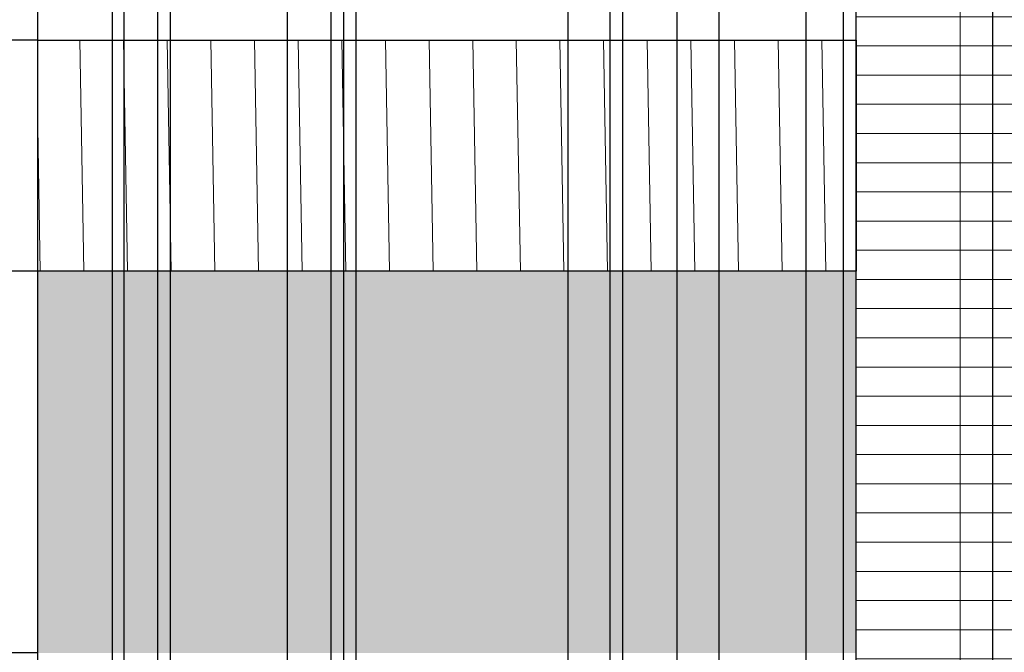
# Model space of a CAD drawing. Units: inches. Extents: x 241 to 943, y 109 to 1396.
# Tile 24 of 34: x 374 to 532, y 1178 to 1279. Entities that reach past the tile are written whole.
import ezdxf

# ---------------------------------------------------------------- set-up
doc = ezdxf.new("R2010")
doc.units = ezdxf.units.IN
doc.header["$MEASUREMENT"] = 0
for name, color, linetype, lineweight in [('A-ANNO-DIMS', 2, 'Continuous', 18), ('A-ELEV', 7, 'Continuous', 25), ('A-ELEV-SHAD', 9, 'Continuous', 13), ('A-WALL-PATT', 8, 'Continuous', 13)]:
    doc.layers.add(name, color=color, linetype=linetype, lineweight=lineweight)
doc.styles.get("Standard").update_dxf_attribs({"font": 'arial.ttf'})
doc.dimstyles.get("Standard").update_dxf_attribs({"dimtxt": 1.4375, "dimasz": 0.18, "dimexe": 0.18, "dimexo": 0.0625, "dimgap": 0.09, "dimtad": 0, "dimtih": 1, "dimtoh": 1, "dimdec": 4, "dimzin": 0, "dimdsep": 46, "dimlunit": 4, "dimtxsty": 'Standard', "dimcen": 0.09, "dimadec": 0, "dimazin": 0, "dimtfac": 1, "dimtdec": 4, "dimtofl": 0, "dimtmove": 0, "dimatfit": 3, "dimfxl": 1, "dimtolj": 1, "dimtzin": 0, "dimarcsym": 0})

# ---------------------------------------------------------------- blocks, each defined once
blk = doc.blocks.new('*D5')
at = {"layer": 'A-ANNO-DIMS', "color": 0, "lineweight": -2, "transparency": 16777216}
for p, q in [((303.24, 177.8), (303.24, 1395.05)), ((303.42, 1394.87), (338.18, 1394.87)), ((376.86, 1394.87), (342.09, 1394.87)), ((377.04, 177.76), (377.04, 1395.05))]:
    blk.add_line(p, q, dxfattribs=at)
at = {"layer": 'A-ANNO-DIMS', "color": 0, "transparency": 16777216}
for points in [[(303.42, 1394.9), (303.42, 1394.84), (303.24, 1394.87)], [(376.86, 1394.9), (376.86, 1394.84), (377.04, 1394.87)]]:
    blk.add_solid(points, dxfattribs=at)
at = {"layer": 'Defpoints', "color": 0, "transparency": 16777216}
for p in [(377.04, 1394.87), (303.24, 177.74), (377.04, 177.7)]:
    blk.add_point(p, dxfattribs=at)
at = {"layer": 'A-ANNO-DIMS', "color": 0, "transparency": 16777216, "insert": (340.14, 1394.87), "char_height": 1.438, "attachment_point": 5}
blk.add_mtext('\\A1;73.8', dxfattribs=at)
blk = doc.blocks.new('*D7')
at = {"layer": 'A-ANNO-DIMS', "color": 0, "lineweight": -2, "transparency": 16777216}
for p, q in [((508.24, 1336.12), (244.31, 1336.12)), ((244.49, 1335.94), (244.49, 753.25)), ((244.49, 168.92), (244.49, 751.6)), ((303.17, 168.74), (244.31, 168.74))]:
    blk.add_line(p, q, dxfattribs=at)
at = {"layer": 'A-ANNO-DIMS', "color": 0, "transparency": 16777216}
for points in [[(244.46, 1335.94), (244.52, 1335.94), (244.49, 1336.12)], [(244.46, 168.92), (244.52, 168.92), (244.49, 168.74)]]:
    blk.add_solid(points, dxfattribs=at)
at = {"layer": 'Defpoints', "color": 0, "transparency": 16777216}
for p in [(244.49, 1336.12), (508.31, 1336.12), (303.24, 168.74)]:
    blk.add_point(p, dxfattribs=at)
at = {"layer": 'A-ANNO-DIMS', "color": 0, "transparency": 16777216, "insert": (244.49, 752.43), "char_height": 1.438, "attachment_point": 5}
blk.add_mtext('\\A1;1167.4', dxfattribs=at)
blk = doc.blocks.new('*D8')
at = {"layer": 'A-ANNO-DIMS', "color": 0, "lineweight": -2, "transparency": 16777216}
for p, q in [((377.04, 396.94), (377.04, 1395.05)), ((377.22, 1394.87), (380.96, 1394.87)), ((390.71, 1394.87), (386.97, 1394.87)), ((390.89, 384.24), (390.89, 1395.05))]:
    blk.add_line(p, q, dxfattribs=at)
at = {"layer": 'A-ANNO-DIMS', "color": 0, "transparency": 16777216}
for points in [[(377.22, 1394.9), (377.22, 1394.84), (377.04, 1394.87)], [(390.71, 1394.9), (390.71, 1394.84), (390.89, 1394.87)]]:
    blk.add_solid(points, dxfattribs=at)
at = {"layer": 'Defpoints', "color": 0, "transparency": 16777216}
for p in [(390.89, 1394.87), (377.04, 396.88), (390.89, 384.18)]:
    blk.add_point(p, dxfattribs=at)
at = {"layer": 'A-ANNO-DIMS', "color": 0, "transparency": 16777216, "insert": (383.97, 1394.87), "char_height": 1.438, "attachment_point": 5}
blk.add_mtext('\\A1;13.856', dxfattribs=at)
blk = doc.blocks.new('*D9')
at = {"layer": 'A-ANNO-DIMS', "color": 0, "lineweight": -2, "transparency": 16777216}
for p, q in [((390.89, 384.24), (390.89, 1395.05)), ((391.07, 1394.87), (424.13, 1394.87)), ((461.93, 1394.87), (428.87, 1394.87)), ((462.11, 384.24), (462.11, 1395.05))]:
    blk.add_line(p, q, dxfattribs=at)
at = {"layer": 'A-ANNO-DIMS', "color": 0, "transparency": 16777216}
for points in [[(391.07, 1394.9), (391.07, 1394.84), (390.89, 1394.87)], [(461.93, 1394.9), (461.93, 1394.84), (462.11, 1394.87)]]:
    blk.add_solid(points, dxfattribs=at)
at = {"layer": 'Defpoints', "color": 0, "transparency": 16777216}
for p in [(462.11, 1394.87), (390.89, 384.18), (462.11, 384.18)]:
    blk.add_point(p, dxfattribs=at)
at = {"layer": 'A-ANNO-DIMS', "color": 0, "transparency": 16777216, "insert": (426.5, 1394.87), "char_height": 1.438, "attachment_point": 5}
blk.add_mtext('\\A1;71.21', dxfattribs=at)
blk = doc.blocks.new('*D10')
at = {"layer": 'A-ANNO-DIMS', "color": 0, "lineweight": -2, "transparency": 16777216}
for p, q in [((462.11, 384.24), (462.11, 1395.05)), ((462.29, 1394.87), (468.4, 1394.87)), ((479.42, 1394.87), (473.3, 1394.87)), ((479.6, 384.24), (479.6, 1395.05))]:
    blk.add_line(p, q, dxfattribs=at)
at = {"layer": 'A-ANNO-DIMS', "color": 0, "transparency": 16777216}
for points in [[(462.29, 1394.9), (462.29, 1394.84), (462.11, 1394.87)], [(479.42, 1394.9), (479.42, 1394.84), (479.6, 1394.87)]]:
    blk.add_solid(points, dxfattribs=at)
at = {"layer": 'Defpoints', "color": 0, "transparency": 16777216}
for p in [(479.6, 1394.87), (462.11, 384.18), (479.6, 384.18)]:
    blk.add_point(p, dxfattribs=at)
at = {"layer": 'A-ANNO-DIMS', "color": 0, "transparency": 16777216, "insert": (470.85, 1394.87), "char_height": 1.438, "attachment_point": 5}
blk.add_mtext('\\A1;17.49', dxfattribs=at)
blk = doc.blocks.new('*D11')
at = {"layer": 'A-ANNO-DIMS', "color": 0, "lineweight": -2, "transparency": 16777216}
for p, q in [((500.33, 384.24), (500.33, 1395.05)), ((500.51, 1394.87), (513.31, 1394.87)), ((530.05, 1394.87), (517.25, 1394.87)), ((530.23, 384.24), (530.23, 1395.05))]:
    blk.add_line(p, q, dxfattribs=at)
at = {"layer": 'A-ANNO-DIMS', "color": 0, "transparency": 16777216}
for points in [[(500.51, 1394.9), (500.51, 1394.84), (500.33, 1394.87)], [(530.05, 1394.9), (530.05, 1394.84), (530.23, 1394.87)]]:
    blk.add_solid(points, dxfattribs=at)
at = {"layer": 'Defpoints', "color": 0, "transparency": 16777216}
for p in [(530.23, 1394.87), (500.33, 384.18), (530.23, 384.18)]:
    blk.add_point(p, dxfattribs=at)
at = {"layer": 'A-ANNO-DIMS', "color": 0, "transparency": 16777216, "insert": (515.28, 1394.87), "char_height": 1.438, "attachment_point": 5}
blk.add_mtext('\\A1;29.9', dxfattribs=at)
blk = doc.blocks.new('*D12')
at = {"layer": 'A-ANNO-DIMS', "color": 0, "lineweight": -2, "transparency": 16777216}
for p, q in [((530.23, 384.24), (530.23, 1395.05)), ((530.41, 1394.87), (587.56, 1394.87)), ((650.73, 1394.87), (593.58, 1394.87)), ((650.91, 384.24), (650.91, 1395.05))]:
    blk.add_line(p, q, dxfattribs=at)
at = {"layer": 'A-ANNO-DIMS', "color": 0, "transparency": 16777216}
for points in [[(530.41, 1394.9), (530.41, 1394.84), (530.23, 1394.87)], [(650.73, 1394.9), (650.73, 1394.84), (650.91, 1394.87)]]:
    blk.add_solid(points, dxfattribs=at)
at = {"layer": 'Defpoints', "color": 0, "transparency": 16777216}
for p in [(650.91, 1394.87), (530.23, 384.18), (650.91, 384.18)]:
    blk.add_point(p, dxfattribs=at)
at = {"layer": 'A-ANNO-DIMS', "color": 0, "transparency": 16777216, "insert": (590.57, 1394.87), "char_height": 1.438, "attachment_point": 5}
blk.add_mtext('\\A1;120.68', dxfattribs=at)
blk = doc.blocks.new('*D17')
at = {"layer": 'A-ANNO-DIMS', "color": 0, "lineweight": -2, "transparency": 16777216}
for p, q in [((377.04, 1275.98), (377.04, 1395.05)), ((377.22, 1394.87), (439.67, 1394.87)), ((508.13, 1394.87), (445.68, 1394.87)), ((508.31, 1275.98), (508.31, 1395.05))]:
    blk.add_line(p, q, dxfattribs=at)
at = {"layer": 'A-ANNO-DIMS', "color": 0, "transparency": 16777216}
for points in [[(377.22, 1394.9), (377.22, 1394.84), (377.04, 1394.87)], [(508.13, 1394.9), (508.13, 1394.84), (508.31, 1394.87)]]:
    blk.add_solid(points, dxfattribs=at)
at = {"layer": 'Defpoints', "color": 0, "transparency": 16777216}
for p in [(508.31, 1394.87), (377.04, 1275.91), (508.31, 1275.91)]:
    blk.add_point(p, dxfattribs=at)
at = {"layer": 'A-ANNO-DIMS', "color": 0, "transparency": 16777216, "insert": (442.67, 1394.87), "char_height": 1.438, "attachment_point": 5}
blk.add_mtext('\\A1;131.27', dxfattribs=at)
blk = doc.blocks.new('*D27')
at = {"layer": 'A-ANNO-DIMS', "color": 0, "lineweight": -2, "transparency": 16777216}
for p, q in [((376.98, 1238.85), (244.31, 1238.85)), ((244.49, 1238.67), (244.49, 1209.02)), ((244.49, 1177.72), (244.49, 1207.37)), ((376.98, 1177.54), (244.31, 1177.54))]:
    blk.add_line(p, q, dxfattribs=at)
at = {"layer": 'A-ANNO-DIMS', "color": 0, "transparency": 16777216}
for points in [[(244.46, 1238.67), (244.52, 1238.67), (244.49, 1238.85)], [(244.46, 1177.72), (244.52, 1177.72), (244.49, 1177.54)]]:
    blk.add_solid(points, dxfattribs=at)
at = {"layer": 'Defpoints', "color": 0, "transparency": 16777216}
for p in [(244.49, 1238.85), (377.04, 1238.85), (377.04, 1177.54)]:
    blk.add_point(p, dxfattribs=at)
at = {"layer": 'A-ANNO-DIMS', "color": 0, "transparency": 16777216, "insert": (244.49, 1208.2), "char_height": 1.438, "attachment_point": 5}
blk.add_mtext('\\A1;61.32', dxfattribs=at)
blk = doc.blocks.new('*D28')
at = {"layer": 'A-ANNO-DIMS', "color": 0, "lineweight": -2, "transparency": 16777216}
for p, q in [((376.98, 1275.91), (244.31, 1275.91)), ((244.49, 1275.73), (244.49, 1258.21)), ((244.49, 1239.03), (244.49, 1256.56)), ((376.98, 1238.85), (244.31, 1238.85))]:
    blk.add_line(p, q, dxfattribs=at)
at = {"layer": 'A-ANNO-DIMS', "color": 0, "transparency": 16777216}
for points in [[(244.46, 1275.73), (244.52, 1275.73), (244.49, 1275.91)], [(244.46, 1239.03), (244.52, 1239.03), (244.49, 1238.85)]]:
    blk.add_solid(points, dxfattribs=at)
at = {"layer": 'Defpoints', "color": 0, "transparency": 16777216}
for p in [(244.49, 1275.91), (377.04, 1275.91), (377.04, 1238.85)]:
    blk.add_point(p, dxfattribs=at)
at = {"layer": 'A-ANNO-DIMS', "color": 0, "transparency": 16777216, "insert": (244.49, 1257.38), "char_height": 1.438, "attachment_point": 5}
blk.add_mtext('\\A1;37.06', dxfattribs=at)
blk = doc.blocks.new('*D57')
at = {"layer": 'A-ANNO-DIMS', "color": 0, "lineweight": -2, "transparency": 16777216}
for p, q in [((508.31, 1070.92), (508.31, 1395.05)), ((508.49, 1394.87), (518.04, 1394.87)), ((533.77, 1394.87), (524.21, 1394.87)), ((533.95, 1108.23), (533.95, 1395.05))]:
    blk.add_line(p, q, dxfattribs=at)
at = {"layer": 'A-ANNO-DIMS', "color": 0, "transparency": 16777216}
for points in [[(508.49, 1394.9), (508.49, 1394.84), (508.31, 1394.87)], [(533.77, 1394.9), (533.77, 1394.84), (533.95, 1394.87)]]:
    blk.add_solid(points, dxfattribs=at)
at = {"layer": 'Defpoints', "color": 0, "transparency": 16777216}
for p in [(533.95, 1394.87), (533.95, 1108.17), (508.31, 1070.85)]:
    blk.add_point(p, dxfattribs=at)
at = {"layer": 'A-ANNO-DIMS', "color": 0, "transparency": 16777216, "insert": (521.13, 1394.87), "char_height": 1.438, "attachment_point": 5}
blk.add_mtext('\\A1;25.646', dxfattribs=at)
blk = doc.blocks.new('*D59')
at = {"layer": 'A-ANNO-DIMS', "color": 0, "lineweight": -2, "transparency": 16777216}
for p, q in [((398.31, 1175.6), (398.31, 1395.05)), ((398.49, 1394.87), (450.7, 1394.87)), ((506.13, 1394.87), (453.92, 1394.87)), ((506.31, 1175.6), (506.31, 1395.05))]:
    blk.add_line(p, q, dxfattribs=at)
at = {"layer": 'A-ANNO-DIMS', "color": 0, "transparency": 16777216}
for points in [[(398.49, 1394.9), (398.49, 1394.84), (398.31, 1394.87)], [(506.13, 1394.9), (506.13, 1394.84), (506.31, 1394.87)]]:
    blk.add_solid(points, dxfattribs=at)
at = {"layer": 'Defpoints', "color": 0, "transparency": 16777216}
for p in [(506.31, 1394.87), (398.31, 1175.54), (506.31, 1175.54)]:
    blk.add_point(p, dxfattribs=at)
at = {"layer": 'A-ANNO-DIMS', "color": 0, "transparency": 16777216, "insert": (452.31, 1394.87), "char_height": 1.438, "attachment_point": 5}
blk.add_mtext('\\A1;108', dxfattribs=at)
blk = doc.blocks.new('*D60')
at = {"layer": 'A-ANNO-DIMS', "color": 0, "lineweight": -2, "transparency": 16777216}
for p, q in [((377.04, 1177.6), (377.04, 1395.05)), ((377.22, 1394.87), (384.59, 1394.87)), ((398.13, 1394.87), (390.76, 1394.87)), ((398.31, 1175.6), (398.31, 1395.05))]:
    blk.add_line(p, q, dxfattribs=at)
at = {"layer": 'A-ANNO-DIMS', "color": 0, "transparency": 16777216}
for points in [[(377.22, 1394.9), (377.22, 1394.84), (377.04, 1394.87)], [(398.13, 1394.9), (398.13, 1394.84), (398.31, 1394.87)]]:
    blk.add_solid(points, dxfattribs=at)
at = {"layer": 'Defpoints', "color": 0, "transparency": 16777216}
for p in [(398.31, 1394.87), (377.04, 1177.54), (398.31, 1175.54)]:
    blk.add_point(p, dxfattribs=at)
at = {"layer": 'A-ANNO-DIMS', "color": 0, "transparency": 16777216, "insert": (387.68, 1394.87), "char_height": 1.438, "attachment_point": 5}
blk.add_mtext('\\A1;21.273', dxfattribs=at)
blk = doc.blocks.new('*D61')
at = {"layer": 'A-ANNO-DIMS', "color": 0, "lineweight": -2, "transparency": 16777216}
for p, q in [((377.04, 400.89), (377.04, 1395.05)), ((377.22, 1394.87), (398.03, 1394.87)), ((423.93, 1394.87), (403.12, 1394.87)), ((424.11, 568.89), (424.11, 1395.05))]:
    blk.add_line(p, q, dxfattribs=at)
at = {"layer": 'A-ANNO-DIMS', "color": 0, "transparency": 16777216}
for points in [[(377.22, 1394.9), (377.22, 1394.84), (377.04, 1394.87)], [(423.93, 1394.9), (423.93, 1394.84), (424.11, 1394.87)]]:
    blk.add_solid(points, dxfattribs=at)
at = {"layer": 'Defpoints', "color": 0, "transparency": 16777216}
for p in [(424.11, 1394.87), (424.11, 568.83), (377.04, 400.83)]:
    blk.add_point(p, dxfattribs=at)
at = {"layer": 'A-ANNO-DIMS', "color": 0, "transparency": 16777216, "insert": (400.57, 1394.87), "char_height": 1.438, "attachment_point": 5}
blk.add_mtext('\\A1;47.07', dxfattribs=at)
blk = doc.blocks.new('*D62')
at = {"layer": 'A-ANNO-DIMS', "color": 0, "lineweight": -2, "transparency": 16777216}
for p, q in [((424.11, 568.89), (424.11, 1395.05)), ((424.29, 1394.87), (492.35, 1394.87)), ((565.02, 1394.87), (496.96, 1394.87)), ((565.2, 568.89), (565.2, 1395.05))]:
    blk.add_line(p, q, dxfattribs=at)
at = {"layer": 'A-ANNO-DIMS', "color": 0, "transparency": 16777216}
for points in [[(424.29, 1394.9), (424.29, 1394.84), (424.11, 1394.87)], [(565.02, 1394.9), (565.02, 1394.84), (565.2, 1394.87)]]:
    blk.add_solid(points, dxfattribs=at)
at = {"layer": 'Defpoints', "color": 0, "transparency": 16777216}
for p in [(565.2, 1394.87), (424.11, 568.83), (565.2, 568.83)]:
    blk.add_point(p, dxfattribs=at)
at = {"layer": 'A-ANNO-DIMS', "color": 0, "transparency": 16777216, "insert": (494.66, 1394.87), "char_height": 1.438, "attachment_point": 5}
blk.add_mtext('\\A1;141.1', dxfattribs=at)
blk = doc.blocks.new('*D65')
at = {"layer": 'A-ANNO-DIMS', "color": 0, "lineweight": -2, "transparency": 16777216}
for p, q in [((424.11, 700.85), (424.11, 1395.05)), ((424.29, 1394.87), (505.52, 1394.87)), ((592.77, 1394.87), (511.54, 1394.87)), ((592.95, 700.85), (592.95, 1395.05))]:
    blk.add_line(p, q, dxfattribs=at)
at = {"layer": 'A-ANNO-DIMS', "color": 0, "transparency": 16777216}
for points in [[(424.29, 1394.9), (424.29, 1394.84), (424.11, 1394.87)], [(592.77, 1394.9), (592.77, 1394.84), (592.95, 1394.87)]]:
    blk.add_solid(points, dxfattribs=at)
at = {"layer": 'Defpoints', "color": 0, "transparency": 16777216}
for p in [(592.95, 1394.87), (424.11, 700.79), (592.95, 700.79)]:
    blk.add_point(p, dxfattribs=at)
at = {"layer": 'A-ANNO-DIMS', "color": 0, "transparency": 16777216, "insert": (508.53, 1394.87), "char_height": 1.438, "attachment_point": 5}
blk.add_mtext('\\A1;168.85', dxfattribs=at)
blk = doc.blocks.new('*D67')
at = {"layer": 'A-ANNO-DIMS', "color": 0, "lineweight": -2, "transparency": 16777216}
for p, q in [((389.04, 773.55), (389.04, 1395.05)), ((389.22, 1394.87), (495.34, 1394.87)), ((607.64, 1394.87), (501.52, 1394.87)), ((607.82, 773.55), (607.82, 1395.05))]:
    blk.add_line(p, q, dxfattribs=at)
at = {"layer": 'A-ANNO-DIMS', "color": 0, "transparency": 16777216}
for points in [[(389.22, 1394.9), (389.22, 1394.84), (389.04, 1394.87)], [(607.64, 1394.9), (607.64, 1394.84), (607.82, 1394.87)]]:
    blk.add_solid(points, dxfattribs=at)
at = {"layer": 'Defpoints', "color": 0, "transparency": 16777216}
for p in [(607.82, 1394.87), (389.04, 773.49), (607.82, 773.49)]:
    blk.add_point(p, dxfattribs=at)
at = {"layer": 'A-ANNO-DIMS', "color": 0, "transparency": 16777216, "insert": (498.43, 1394.87), "char_height": 1.438, "attachment_point": 5}
blk.add_mtext('\\A1;218.77', dxfattribs=at)
blk = doc.blocks.new('*D69')
at = {"layer": 'A-ANNO-DIMS', "color": 0, "lineweight": -2, "transparency": 16777216}
for p, q in [((389.04, 941.55), (389.04, 1395.05)), ((389.22, 1394.87), (476.28, 1394.87)), ((567.95, 1394.87), (480.9, 1394.87)), ((568.13, 941.55), (568.13, 1395.05))]:
    blk.add_line(p, q, dxfattribs=at)
at = {"layer": 'A-ANNO-DIMS', "color": 0, "transparency": 16777216}
for points in [[(389.22, 1394.9), (389.22, 1394.84), (389.04, 1394.87)], [(567.95, 1394.9), (567.95, 1394.84), (568.13, 1394.87)]]:
    blk.add_solid(points, dxfattribs=at)
at = {"layer": 'Defpoints', "color": 0, "transparency": 16777216}
for p in [(568.13, 1394.87), (389.04, 941.49), (568.13, 941.49)]:
    blk.add_point(p, dxfattribs=at)
at = {"layer": 'A-ANNO-DIMS', "color": 0, "transparency": 16777216, "insert": (478.59, 1394.87), "char_height": 1.438, "attachment_point": 5}
blk.add_mtext('\\A1;179.1', dxfattribs=at)
blk = doc.blocks.new('*D72')
at = {"layer": 'A-ANNO-DIMS', "color": 0, "lineweight": -2, "transparency": 16777216}
for p, q in [((389.04, 1109.55), (389.04, 1395.05)), ((389.22, 1394.87), (435.74, 1394.87)), ((486.16, 1394.87), (439.65, 1394.87)), ((486.34, 1109.55), (486.34, 1395.05))]:
    blk.add_line(p, q, dxfattribs=at)
at = {"layer": 'A-ANNO-DIMS', "color": 0, "transparency": 16777216}
for points in [[(389.22, 1394.9), (389.22, 1394.84), (389.04, 1394.87)], [(486.16, 1394.9), (486.16, 1394.84), (486.34, 1394.87)]]:
    blk.add_solid(points, dxfattribs=at)
at = {"layer": 'Defpoints', "color": 0, "transparency": 16777216}
for p in [(486.34, 1394.87), (389.04, 1109.49), (486.34, 1109.49)]:
    blk.add_point(p, dxfattribs=at)
at = {"layer": 'A-ANNO-DIMS', "color": 0, "transparency": 16777216, "insert": (437.69, 1394.87), "char_height": 1.438, "attachment_point": 5}
blk.add_mtext('\\A1;97.3', dxfattribs=at)
blk = doc.blocks.new('*D79')
at = {"layer": 'A-ANNO-DIMS', "color": 0, "lineweight": -2, "transparency": 16777216}
for p, q in [((479.6, 384.24), (479.6, 1395.05)), ((479.78, 1394.87), (486.88, 1394.87)), ((500.15, 1394.87), (493.05, 1394.87)), ((500.33, 384.24), (500.33, 1395.05))]:
    blk.add_line(p, q, dxfattribs=at)
at = {"layer": 'A-ANNO-DIMS', "color": 0, "transparency": 16777216}
for points in [[(479.78, 1394.9), (479.78, 1394.84), (479.6, 1394.87)], [(500.15, 1394.9), (500.15, 1394.84), (500.33, 1394.87)]]:
    blk.add_solid(points, dxfattribs=at)
at = {"layer": 'Defpoints', "color": 0, "transparency": 16777216}
for p in [(500.33, 1394.87), (479.6, 384.18), (500.33, 384.18)]:
    blk.add_point(p, dxfattribs=at)
at = {"layer": 'A-ANNO-DIMS', "color": 0, "transparency": 16777216, "insert": (489.96, 1394.87), "char_height": 1.438, "attachment_point": 5}
blk.add_mtext('\\A1;20.736', dxfattribs=at)
blk = doc.blocks.new('*D89')
at = {"layer": 'A-ANNO-DIMS', "color": 0, "lineweight": -2, "transparency": 16777216}
for p, q in [((377.04, 841.6), (377.04, 1395.05)), ((377.22, 1394.87), (494.32, 1394.87)), ((617.58, 1394.87), (500.48, 1394.87)), ((617.76, 841.6), (617.76, 1395.05))]:
    blk.add_line(p, q, dxfattribs=at)
at = {"layer": 'A-ANNO-DIMS', "color": 0, "transparency": 16777216}
for points in [[(377.22, 1394.9), (377.22, 1394.84), (377.04, 1394.87)], [(617.58, 1394.9), (617.58, 1394.84), (617.76, 1394.87)]]:
    blk.add_solid(points, dxfattribs=at)
at = {"layer": 'Defpoints', "color": 0, "transparency": 16777216}
for p in [(617.76, 1394.87), (377.04, 841.54), (617.76, 841.54)]:
    blk.add_point(p, dxfattribs=at)
at = {"layer": 'A-ANNO-DIMS', "color": 0, "transparency": 16777216, "insert": (497.4, 1394.87), "char_height": 1.438, "attachment_point": 5}
blk.add_mtext('\\A1;240.72', dxfattribs=at)
blk = doc.blocks.new('*D92')
at = {"layer": 'A-ANNO-DIMS', "color": 0, "lineweight": -2, "transparency": 16777216}
for p, q in [((508.24, 1336.12), (244.31, 1336.12)), ((244.49, 1335.94), (244.49, 1204.31)), ((244.49, 1071.03), (244.49, 1202.66)), ((508.24, 1070.85), (244.31, 1070.85))]:
    blk.add_line(p, q, dxfattribs=at)
at = {"layer": 'A-ANNO-DIMS', "color": 0, "transparency": 16777216}
for points in [[(244.46, 1335.94), (244.52, 1335.94), (244.49, 1336.12)], [(244.46, 1071.03), (244.52, 1071.03), (244.49, 1070.85)]]:
    blk.add_solid(points, dxfattribs=at)
at = {"layer": 'Defpoints', "color": 0, "transparency": 16777216}
for p in [(244.49, 1336.12), (508.31, 1336.12), (508.31, 1070.85)]:
    blk.add_point(p, dxfattribs=at)
at = {"layer": 'A-ANNO-DIMS', "color": 0, "transparency": 16777216, "insert": (244.49, 1203.48), "char_height": 1.438, "attachment_point": 5}
blk.add_mtext('\\A1;265.26', dxfattribs=at)
blk = doc.blocks.new('*D99')
at = {"layer": 'A-ANNO-DIMS', "color": 0, "lineweight": -2, "transparency": 16777216}
for p, q in [((417.09, 181.71), (417.09, 1395.05)), ((417.27, 1394.87), (539.16, 1394.87)), ((667.21, 1394.87), (545.33, 1394.87)), ((667.39, 214.58), (667.39, 1395.05))]:
    blk.add_line(p, q, dxfattribs=at)
at = {"layer": 'A-ANNO-DIMS', "color": 0, "transparency": 16777216}
for points in [[(417.27, 1394.9), (417.27, 1394.84), (417.09, 1394.87)], [(667.21, 1394.9), (667.21, 1394.84), (667.39, 1394.87)]]:
    blk.add_solid(points, dxfattribs=at)
at = {"layer": 'Defpoints', "color": 0, "transparency": 16777216}
for p in [(667.39, 1394.87), (667.39, 214.52), (417.09, 181.65)]:
    blk.add_point(p, dxfattribs=at)
at = {"layer": 'A-ANNO-DIMS', "color": 0, "transparency": 16777216, "insert": (542.24, 1394.87), "char_height": 1.438, "attachment_point": 5}
blk.add_mtext('\\A1;250.30', dxfattribs=at)
blk = doc.blocks.new('*D101')
at = {"layer": 'A-ANNO-DIMS', "color": 0, "lineweight": -2, "transparency": 16777216}
for p, q in [((396.31, 1009.6), (396.31, 1395.05)), ((396.49, 1394.87), (408.12, 1394.87)), ((425.94, 1394.87), (414.31, 1394.87)), ((426.12, 1007.6), (426.12, 1395.05))]:
    blk.add_line(p, q, dxfattribs=at)
at = {"layer": 'A-ANNO-DIMS', "color": 0, "transparency": 16777216}
for points in [[(396.49, 1394.9), (396.49, 1394.84), (396.31, 1394.87)], [(425.94, 1394.9), (425.94, 1394.84), (426.12, 1394.87)]]:
    blk.add_solid(points, dxfattribs=at)
at = {"layer": 'Defpoints', "color": 0, "transparency": 16777216}
for p in [(426.12, 1394.87), (396.31, 1009.54), (426.12, 1007.54)]:
    blk.add_point(p, dxfattribs=at)
at = {"layer": 'A-ANNO-DIMS', "color": 0, "transparency": 16777216, "insert": (411.21, 1394.87), "char_height": 1.438, "attachment_point": 5}
blk.add_mtext('\\A1;29.805', dxfattribs=at)
blk = doc.blocks.new('*D102')
at = {"layer": 'A-ANNO-DIMS', "color": 0, "lineweight": -2, "transparency": 16777216}
for p, q in [((428.12, 1007.6), (428.12, 1395.05)), ((428.3, 1394.87), (445.94, 1394.87)), ((468.69, 1394.87), (451.04, 1394.87)), ((468.87, 1007.6), (468.87, 1395.05))]:
    blk.add_line(p, q, dxfattribs=at)
at = {"layer": 'A-ANNO-DIMS', "color": 0, "transparency": 16777216}
for points in [[(428.3, 1394.9), (428.3, 1394.84), (428.12, 1394.87)], [(468.69, 1394.9), (468.69, 1394.84), (468.87, 1394.87)]]:
    blk.add_solid(points, dxfattribs=at)
at = {"layer": 'Defpoints', "color": 0, "transparency": 16777216}
for p in [(468.87, 1394.87), (428.12, 1007.54), (468.87, 1007.54)]:
    blk.add_point(p, dxfattribs=at)
at = {"layer": 'A-ANNO-DIMS', "color": 0, "transparency": 16777216, "insert": (448.49, 1394.87), "char_height": 1.438, "attachment_point": 5}
blk.add_mtext('\\A1;40.75', dxfattribs=at)
blk = doc.blocks.new('*D103')
at = {"layer": 'A-ANNO-DIMS', "color": 0, "lineweight": -2, "transparency": 16777216}
for p, q in [((470.87, 1007.6), (470.87, 1395.05)), ((471.05, 1394.87), (487.08, 1394.87)), ((508.13, 1394.87), (492.1, 1394.87)), ((508.31, 1009.6), (508.31, 1395.05))]:
    blk.add_line(p, q, dxfattribs=at)
at = {"layer": 'A-ANNO-DIMS', "color": 0, "transparency": 16777216}
for points in [[(471.05, 1394.9), (471.05, 1394.84), (470.87, 1394.87)], [(508.13, 1394.9), (508.13, 1394.84), (508.31, 1394.87)]]:
    blk.add_solid(points, dxfattribs=at)
at = {"layer": 'Defpoints', "color": 0, "transparency": 16777216}
for p in [(508.31, 1394.87), (508.31, 1009.54), (470.87, 1007.54)]:
    blk.add_point(p, dxfattribs=at)
at = {"layer": 'A-ANNO-DIMS', "color": 0, "transparency": 16777216, "insert": (489.59, 1394.87), "char_height": 1.438, "attachment_point": 5}
blk.add_mtext('\\A1;37.44', dxfattribs=at)

msp = doc.modelspace()

# ---------------------------------------------------------------- hatches: boundary and pattern name
at = {"layer": 'A-ELEV-SHAD'}
h = msp.add_hatch(color=256, dxfattribs=at)
h.dxf.hatch_style = 1
h.paths.add_polyline_path([(508.3064, 1070.8538), (377.0391, 1070.8538), (377.0391, 1009.5382), (508.3064, 1009.5382)])
h.paths.add_polyline_path([(508.3064, 1238.8538), (377.0391, 1238.8538), (377.0391, 1177.5382), (508.3064, 1177.5382)])
h.paths.add_polyline_path([(581.3632, 902.8538), (568.1348, 902.8538), (553.5166, 902.8538), (377.0391, 902.8538), (377.0391, 841.5382), (553.5166, 841.5382), (564.8076, 841.5382), (581.3632, 841.5382)])
h.paths.add_polyline_path([(820.8374, 1275.9142), (747.7579, 1275.9142), (747.7579, 1238.8538), (820.8374, 1238.8538)])
h.paths.add_polyline_path([(820.8374, 1238.8538), (747.7579, 1238.8538), (747.9341, 1223.0633), (820.8374, 1223.0633)])
h.paths.add_polyline_path([(396.3125, 841.5382), (377.0391, 841.5382), (377.0391, 734.8538), (389.0429, 734.8538), (389.0429, 735.188), (389.0429, 773.4916), (396.3125, 773.4916), (396.3125, 780.5808), (390.5597, 780.5808), (388.0428, 780.5808, -1), (388.0428, 782.5808), (390.5597, 782.5808), (396.3125, 782.5808)])
at = {"layer": 'A-WALL-PATT'}
h = msp.add_hatch(dxfattribs=at)
h.set_pattern_fill('GRATE', color=256, scale=150)
h.paths.add_polyline_path([(747.7579, 1238.8538), (747.7579, 1275.9142), (747.7579, 1336.1154), (508.3064, 1336.1154), (508.3064, 1275.9142), (508.3064, 1238.8538), (508.3064, 1177.5382), (508.3064, 1109.4916), (508.3064, 1070.8538), (553.5166, 1070.8538), (749.6328, 1070.8538)])
h.paths.add_polyline_path([(533.952, 1108.1686), (533.952, 1177.7336), (533.952, 1303.0286), (724.819, 1303.0286), (724.819, 1108.1686)], flags=16)
h.paths.add_polyline_path([(535.952, 1110.1686), (535.952, 1175.7336), (722.819, 1175.7336), (722.819, 1110.1686)], flags=0)
h.paths.add_polyline_path([(643.4534, 1134.0739), (622.521, 1134.0739), (622.521, 1136.0739), (643.4534, 1136.0739)], flags=0)
h.paths.add_polyline_path([(617.7594, 568.8295), (617.7594, 734.8538), (377.0391, 734.8538), (377.0391, 566.8538), (377.0391, 400.8295), (417.0913, 400.8295), (618.9643, 400.8295)])
h.paths.add_polyline_path([(424.1086, 496.4395), (424.1086, 568.8295), (565.2023, 568.8295), (565.2023, 496.4395)], flags=16)
h.paths.add_polyline_path([(426.1086, 498.4395), (426.1086, 566.8295), (563.2023, 566.8295), (563.2023, 508.9074), (563.2023, 498.4395)], flags=0)
h.paths.add_polyline_path([(508.0803, 508.9074), (508.0803, 519.3754), (450.9259, 519.3754), (450.9259, 525.3816), (445.5808, 525.3816, -1), (445.5808, 527.3816), (450.9259, 527.3816), (450.9259, 566.8295), (508.0803, 566.8295), (537.4269, 566.8295), (537.4269, 508.9074)], flags=0)
h.paths.add_polyline_path([(506.0803, 521.3754), (452.9259, 521.3754), (452.9259, 564.8295), (506.0803, 564.8295)], flags=0)
h.paths.add_polyline_path([(424.1086, 628.4013), (424.1086, 700.7912), (592.9542, 700.7912), (592.9542, 628.4013)], flags=16)
h.paths.add_polyline_path([(426.1086, 630.4013), (426.1086, 698.7912), (590.8792, 698.7912), (590.8792, 630.4013)], flags=0)
h.paths.add_polyline_path([(508.1906, 651.3371), (508.0803, 651.3371), (450.9259, 651.3371), (428.0291, 651.3371), (428.0291, 698.7912), (451.9767, 698.7912), (508.0803, 698.7912), (537.4269, 698.7912), (563.2023, 698.7912), (563.2023, 659.3434), (563.9297, 659.3434), (563.9297, 651.3371)], flags=0)
h.paths.add_polyline_path([(506.0803, 653.3371), (452.9259, 653.3371), (452.9259, 657.3434), (445.5808, 657.3434, -1), (445.5808, 659.3434), (452.9259, 659.3434), (452.9259, 696.7912), (506.0803, 696.7912)], flags=0)
h = msp.add_hatch(dxfattribs=at)
h.set_pattern_fill('ANSI31', color=256, scale=56, angle=46)
h.paths.add_polyline_path([(508.3064, 1275.9142), (377.0391, 1275.9142), (377.0391, 1238.8538), (508.3064, 1238.8538)])
h.paths.add_polyline_path([(724.819, 1237.0695), (533.952, 1237.0695), (533.952, 1177.7336), (724.819, 1177.7336)])

# ---------------------------------------------------------------- linework, layer by layer
at = {"layer": 'A-ELEV'}
for p, q in [((508.3064, 1275.9142), (508.3064, 1336.1154)), ((377.0391, 1238.8538), (377.0391, 1275.9142)), ((377.0391, 1275.9142), (508.3064, 1275.9142)), ((508.3064, 1275.9142), (508.3064, 1238.8538)), ((377.0391, 1070.8538), (377.0391, 1238.8538)), ((508.3064, 1238.8538), (377.0391, 1238.8538)), ((508.3064, 1177.5382), (508.3064, 1238.8538))]:
    msp.add_line(p, q, dxfattribs=at)

# ---------------------------------------------------------------- dimensions: what is measured, and where the dimension line sits
at = {"layer": 'A-ANNO-DIMS'}
for base, p1, p2, override, picture, middle in [((377.0391, 1394.8654), (303.2358, 177.7407), (377.0391, 177.6977), {"dimdec": 1, "dimlfac": 1, "dimrnd": 0, "dimzin": 0, "dimdsep": 46, "dimlunit": 2}, '*D5', (340.1375, 1394.8654)), ((390.895, 1394.8654), (377.0391, 396.8782), (390.895, 384.1784), {"dimdec": 3, "dimlfac": 1, "dimrnd": 0, "dimzin": 0, "dimdsep": 46, "dimlunit": 2}, '*D8', (383.9671, 1394.8654)), ((508.3064, 1394.8654), (377.0391, 1275.9142), (508.3064, 1275.9142), {"dimdec": 2, "dimlfac": 1, "dimrnd": 0, "dimzin": 0, "dimdsep": 46, "dimlunit": 2}, '*D17', (442.6728, 1394.8654)), ((398.3125, 1394.8654), (377.0391, 1177.5382), (398.3125, 1175.5382), {"dimdec": 3, "dimlfac": 1, "dimrnd": 0, "dimzin": 0, "dimdsep": 46, "dimlunit": 2}, '*D60', (387.6758, 1394.8654)), ((424.1086, 1394.8654), (377.0391, 400.8295), (424.1086, 568.8295), {"dimdec": 2, "dimlfac": 1, "dimrnd": 0, "dimzin": 0, "dimdsep": 46, "dimlunit": 2}, '*D61', (400.5739, 1394.8654)), ((617.7594, 1394.8654), (377.0391, 841.5382), (617.7594, 841.5382), {"dimdec": 2, "dimlfac": 1, "dimrnd": 0, "dimzin": 0, "dimdsep": 46, "dimlunit": 2}, '*D89', (497.3993, 1394.8654)), ((607.8162, 1394.8654), (389.0429, 773.4916), (607.8162, 773.4916), {"dimdec": 2, "dimlfac": 1, "dimrnd": 0, "dimzin": 0, "dimdsep": 46, "dimlunit": 2}, '*D67', (498.4295, 1394.8654)), ((568.1348, 1394.8654), (389.0429, 941.4916), (568.1348, 941.4916), {"dimdec": 1, "dimlfac": 1, "dimrnd": 0, "dimzin": 0, "dimdsep": 46, "dimlunit": 2}, '*D69', (478.5888, 1394.8654)), ((486.3418, 1394.8654), (389.0429, 1109.4916), (486.3418, 1109.4916), {"dimdec": 1, "dimlfac": 1, "dimrnd": 0, "dimzin": 0, "dimdsep": 46, "dimlunit": 2}, '*D72', (437.6924, 1394.8654)), ((462.1074, 1394.8654), (390.895, 384.1784), (462.1074, 384.1784), {"dimdec": 2, "dimlfac": 1, "dimrnd": 0, "dimzin": 0, "dimdsep": 46, "dimlunit": 2}, '*D9', (426.5012, 1394.8654)), ((426.1173, 1394.8654), (396.3125, 1009.5382), (426.1173, 1007.5382), {"dimdec": 3, "dimlfac": 1, "dimrnd": 0, "dimzin": 0, "dimdsep": 46, "dimlunit": 2}, '*D101', (411.2149, 1394.8654)), ((506.3064, 1394.8654), (398.3125, 1175.5382), (506.3064, 1175.5382), {"dimdec": 0, "dimlfac": 1, "dimrnd": 0, "dimzin": 0, "dimdsep": 46, "dimlunit": 2}, '*D59', (452.3095, 1394.8654)), ((667.3935, 1394.8654), (417.0913, 181.649), (667.3935, 214.5189), {"dimdec": 2, "dimlfac": 1, "dimrnd": 0, "dimzin": 0, "dimdsep": 46, "dimlunit": 2}, '*D99', (542.2424, 1394.8654)), ((565.2023, 1394.8654), (424.1086, 568.8295), (565.2023, 568.8295), {"dimdec": 1, "dimlfac": 1, "dimrnd": 0, "dimzin": 0, "dimdsep": 46, "dimlunit": 2}, '*D62', (494.6554, 1394.8654)), ((592.9542, 1394.8654), (424.1086, 700.7912), (592.9542, 700.7912), {"dimdec": 2, "dimlfac": 1, "dimrnd": 0, "dimzin": 0, "dimdsep": 46, "dimlunit": 2}, '*D65', (508.5314, 1394.8654)), ((468.8692, 1394.8654), (428.1173, 1007.5382), (468.8692, 1007.5382), {"dimdec": 2, "dimlfac": 1, "dimrnd": 0, "dimzin": 0, "dimdsep": 46, "dimlunit": 2}, '*D102', (448.4933, 1394.8654)), ((479.596, 1394.8654), (462.1074, 384.1784), (479.596, 384.1784), {"dimdec": 2, "dimlfac": 1, "dimrnd": 0, "dimzin": 0, "dimdsep": 46, "dimlunit": 2}, '*D10', (470.8517, 1394.8654)), ((508.3064, 1394.8654), (470.8692, 1007.5382), (508.3064, 1009.5382), {"dimdec": 2, "dimlfac": 1, "dimrnd": 0, "dimzin": 0, "dimdsep": 46, "dimlunit": 2}, '*D103', (489.5878, 1394.8654)), ((500.3323, 1394.8654), (479.596, 384.1784), (500.3323, 384.1784), {"dimdec": 3, "dimlfac": 1, "dimrnd": 0, "dimzin": 0, "dimdsep": 46, "dimlunit": 2}, '*D79', (489.9641, 1394.8654)), ((530.2303, 1394.8654), (500.3323, 384.1784), (530.2303, 384.1784), {"dimdec": 1, "dimlfac": 1, "dimrnd": 0, "dimzin": 0, "dimdsep": 46, "dimlunit": 2}, '*D11', (515.2813, 1394.8654)), ((533.952, 1394.8654), (508.3064, 1070.8538), (533.952, 1108.1686), {"dimdec": 3, "dimlfac": 1, "dimrnd": 0, "dimzin": 0, "dimdsep": 46, "dimlunit": 2}, '*D57', (521.1292, 1394.8654)), ((650.907, 1394.8654), (530.2303, 384.1784), (650.907, 384.1784), {"dimdec": 2, "dimlfac": 1, "dimrnd": 0, "dimzin": 0, "dimdsep": 46, "dimlunit": 2}, '*D12', (590.5686, 1394.8654))]:
    dim = msp.add_linear_dim(base=base, p1=p1, p2=p2, dimstyle='Standard', override=override, dxfattribs=at)
    dim.commit()
    dim.dimension.update_dxf_attribs({"geometry": picture, "text_midpoint": middle})
for base, p1, p2, override, picture, middle in [((244.4858, 1336.1154), (303.2358, 168.7407), (508.3064, 1336.1154), {"dimdec": 1, "dimlfac": 1, "dimrnd": 0, "dimzin": 0, "dimdsep": 46, "dimlunit": 2}, '*D7', (244.4858, 752.4281)), ((244.4858, 1336.1154), (508.3064, 1070.8538), (508.3064, 1336.1154), {"dimdec": 2, "dimlfac": 1, "dimrnd": 0, "dimzin": 0, "dimdsep": 46, "dimlunit": 2}, '*D92', (244.4858, 1203.4846)), ((244.4858, 1275.9142), (377.0391, 1238.8538), (377.0391, 1275.9142), {"dimdec": 2, "dimlfac": 1, "dimrnd": 0, "dimzin": 0, "dimdsep": 46, "dimlunit": 2}, '*D28', (244.4858, 1257.384)), ((244.4858, 1238.8538), (377.0391, 1177.5382), (377.0391, 1238.8538), {"dimdec": 2, "dimlfac": 1, "dimrnd": 0, "dimzin": 0, "dimdsep": 46, "dimlunit": 2}, '*D27', (244.4858, 1208.196))]:
    dim = msp.add_linear_dim(base=base, p1=p1, p2=p2, angle=90, dimstyle='Standard', override=override, dxfattribs=at)
    dim.commit()
    dim.dimension.update_dxf_attribs({"geometry": picture, "text_midpoint": middle})

doc.saveas('drawing.dxf')
